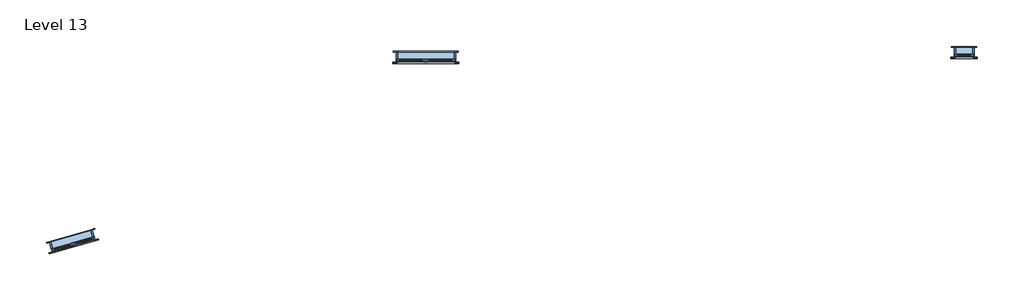
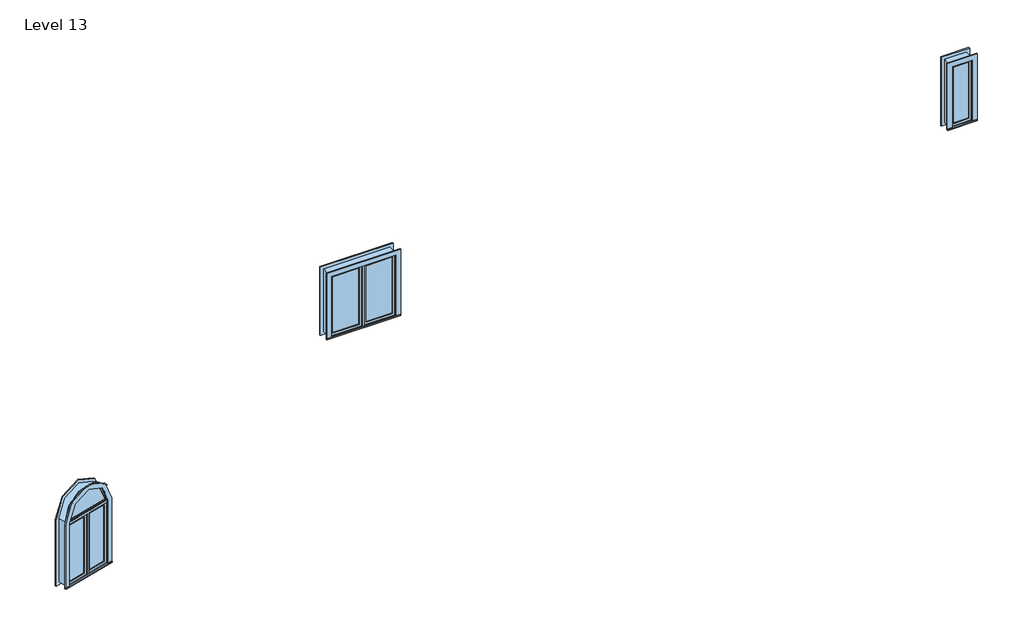
# One storey: 3 windows.
"""IFC4 building model written with IfcOpenShell, lengths in millimetres."""

from ifc_helpers import new_model, si_unit, origin, place, context, project, spatial, transform, mapped, element, save
from components import window_cf4adaea, window_a765b88f, window_0862ab64

model = new_model("IFC4")

# Units and contexts
model_context = context("Model", 3, world=origin())
ifc_project = project(units=[si_unit("LENGTHUNIT", "METRE", prefix="MILLI")], contexts=[model_context])

# Site, building, storey
site = spatial("IfcSite", under=ifc_project)
building = spatial("IfcBuilding", under=site)
storey = spatial("IfcBuildingStorey", under=building, Name="Level 13", Elevation=22860.0)

# Windows
placement = place(None, origin())
window_shape = window_cf4adaea(model_context)
element("IfcWindow", 1, ObjectType="36\" x 48\"", at=placement, inside=storey, context=model_context, shape_type="MappedRepresentation", body=[
    mapped(window_shape, transform((2828.9670453, -16230.7309096, 22860.0), x_axis=(-0.9612486995128053, -0.2756826757069447, 0.0), y_axis=(0.2756826757069447, -0.9612486995128053, 0.0), z_axis=(0.0, 0.0, 1.0))),
])
window_2_shape = window_a765b88f(model_context)
element("IfcWindow", 2, ObjectType="Awning with Trim : 16\" x 48\"", at=placement, inside=storey, context=model_context, shape_type="MappedRepresentation", body=[
    mapped(window_2_shape, transform((21121.014721, -12354.7237084, 22860.0), x_axis=(-1.0, 0.0, 0.0), y_axis=(0.0, -1.0, 0.0), z_axis=(0.0, 0.0, 1.0))),
])
window_3_shape = window_0862ab64(model_context)
element("IfcWindow", 3, ObjectType="Casement Dbl with Trim : 48\" x 48\"", at=placement, inside=storey, context=model_context, shape_type="MappedRepresentation", body=[
    mapped(window_3_shape, transform((10076.7594464, -12437.2737084, 22860.0), x_axis=(-1.0, 0.0, 0.0), y_axis=(0.0, -1.0, 0.0), z_axis=(0.0, 0.0, 1.0))),
])

save(model, "model.ifc")

# Revit data of these elements
# Type "36\" x 48\""
#   Type Mark = "38"
#   Construction Type Id = "SGL"
#   Assembly Code = "B2020100"
#   Analytic Construction = "Large single-glazed windows"
#   Visual Light Transmittance = 0.9
#   Solar Heat Gain Coefficient = 0.86
#   Heat Transfer Coefficient (U) = 0.979472 BTU/(h·ft²·°F)
#   Height = 4' - 0"
#   Default Sill Height = 3' - 0"
#   Trim Projection - Ext. = 0' - 0 1/2"
#   Trim Projection - Int. = 0' - 0 3/4"
#   Trim Width - Exterior = 0' - 3 1/2"
#   Trim Width - Interior = 0' - 3 1/2"
#   Width = 3' - 0"
#   Window Inset = 0' - 0 3/4"
#   Define Thermal Properties by = 1
#   Glass Pane Material = Glass
#   Sash Material = Sash
#   Trim Exterior Material = Trim
#   Trim Interior Material = Trim
#   Wall Closure = (empty or 0)
# Type "Awning with Trim : 16\" x 48\""
#   Type Mark = "14"
#   Construction Type Id = "GSP4R"
#   Assembly Code = "B2020100"
#   Analytic Construction = "1/8 in Pilkington single glazing"
#   Visual Light Transmittance = 0.9
#   Solar Heat Gain Coefficient = 0.78
#   Heat Transfer Coefficient (U) = 0.6496 BTU/(h·ft²·°F)
#   Height = 4' - 0"
#   Default Sill Height = 3' - 0"
#   Trim Projection - Ext. = 0' - 0 1/2"
#   Trim Projection - Int. = 0' - 0 3/4"
#   Trim Width - Exterior = 0' - 3 1/2"
#   Trim Width - Interior = 0' - 3 1/2"
#   Width = 1' - 4"
#   Window Inset = 0' - 0 3/4"
#   Define Thermal Properties by = 1
#   Glass Pane Material = Glass
#   Sash Material = Sash
#   Trim Exterior Material = Trim
#   Trim Interior Material = Trim
#   Wall Closure = (empty or 0)
# Type "Casement Dbl with Trim : 48\" x 48\""
#   Type Mark = "34"
#   Construction Type Id = "GSP4R"
#   Assembly Code = "B2020100"
#   Analytic Construction = "1/8 in Pilkington single glazing"
#   Visual Light Transmittance = 0.9
#   Solar Heat Gain Coefficient = 0.78
#   Heat Transfer Coefficient (U) = 0.6496 BTU/(h·ft²·°F)
#   Height = 4' - 0"
#   Default Sill Height = 3' - 0"
#   Trim Projection - Ext. = 0' - 0 1/2"
#   Trim Projection - Int. = 0' - 0 3/4"
#   Trim Width - Exterior = 0' - 3 1/2"
#   Trim Width - Interior = 0' - 3 1/2"
#   Width = 4' - 0"
#   Window Inset = 0' - 0 3/4"
#   Define Thermal Properties by = 1
#   Glass Pane Material = Glass
#   Sash Material = Sash
#   Trim Exterior Material = Trim
#   Trim Interior Material = Trim
#   Wall Closure = (empty or 0)
# Element 1 (IfcWindow, "36\" x 48\"")
#   Mark = "27"
#   Phase Created = New Construction
#   Materials on its faces: "Sash", "Trim", "Glass"
# Element 2 (IfcWindow, "Awning with Trim : 16\" x 48\"")
#   Mark = "61"
#   Phase Created = New Construction
#   Materials on its faces: "Sash", "Trim", "Glass"
# Element 3 (IfcWindow, "Casement Dbl with Trim : 48\" x 48\"")
#   Mark = "10"
#   Phase Created = New Construction
#   Materials on its faces: "Sash", "Trim", "Glass"
# Materials
#   "Glass": class "Glass", colour RGB 0 128 192, transparency 0.75, Description = "Soda Lime Glass", Cost = 0
#   "Sash": class "Wood", colour RGB 224 178 126, transparency 0
#   "Trim": class "Wood", colour RGB 224 178 126, transparency 0
